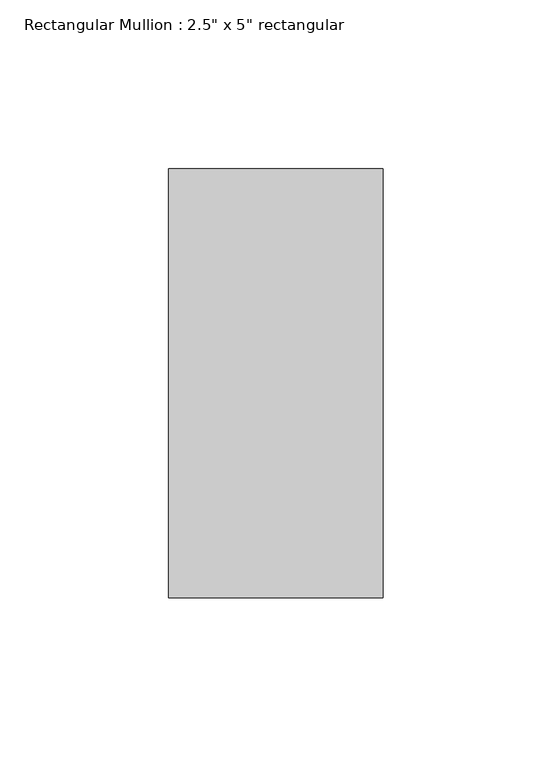
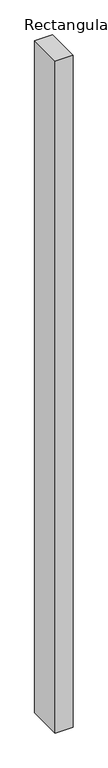
"""IFC4 building model written with IfcOpenShell, lengths in millimetres: member geometry."""

from ifc_helpers import new_model, si_unit, frame, origin, place, context, project, spatial, polyline, outline, extrude, source, transform, mapped, element, save


def member_0aac9e43(model_context):
    return source(origin(), model_context, "Body", "SweptSolid", [
        extrude(outline(polyline([(31.75, 63.5), (31.75, -63.5), (-31.75, -63.5), (-31.75, 63.5), (31.75, 63.5)])), frame((0.0, 0.0, -2529.4963211), z_axis=(0.0, 0.0, 1.0), x_axis=(1.0, 0.0, 0.0)), (0.0, 0.0, 1.0), 2529.4963211),
    ])


if __name__ == "__main__":
    model = new_model("IFC4")
    model_context = context("Model", 3, world=origin())
    ifc_project = project(units=[si_unit("LENGTHUNIT", "METRE", prefix="MILLI")], contexts=[model_context])
    site = spatial("IfcSite", under=ifc_project)
    building = spatial("IfcBuilding", under=site)
    placement = place(None, origin())
    member_shape = member_0aac9e43(model_context)
    element("IfcMember", 1, ObjectType="Rectangular Mullion : 2.5\" x 5\" rectangular", at=placement, inside=building, context=model_context, shape_type="MappedRepresentation", body=[
        mapped(member_shape, transform((0.0, 0.0, 0.0), x_axis=(1.0, 0.0, 0.0), y_axis=(0.0, 1.0, 0.0), z_axis=(0.0, 0.0, 1.0))),
    ])
    save(model, "model.ifc")

# Revit data of these elements
# Type "Rectangular Mullion : 2.5\" x 5\" rectangular"
#   built-in parameter 1007304 = 0.416667 (stored number, unit not read)
#   built-in parameter 1007301 = 0.104167 (stored number, unit not read)
#   built-in parameter 1007300 = 0.104167 (stored number, unit not read)
# Element 1 (IfcMember, "Rectangular Mullion : 2.5\" x 5\" rectangular")
#   Materials on its faces: "Aluminum"
# Materials
#   "Aluminum": class "Metal", colour RGB 247 247 247, transparency 0, Description = "Aluminum 6061", Cost = 0
